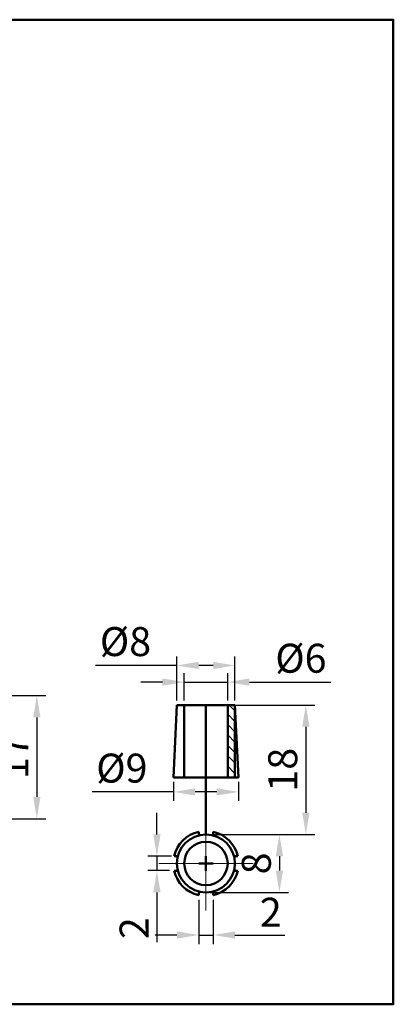
# Model space of a CAD drawing. Units: millimetres. Extents: x 139 to 291, y 28 to 164.
# Tile 5 of 5: x 240 to 291, y 28 to 164. Entities that reach past the tile are written whole.
import ezdxf

# ---------------------------------------------------------------- set-up
doc = ezdxf.new("R2010")
doc.units = ezdxf.units.MM
doc.linetypes.add('CENTER2', pattern=[28.575, 19.05, -3.175, 3.175, -3.175])
for name, color, linetype, lineweight in [('M-CNTR', 1, 'CENTER2', 18), ('M-DIMS', 2, 'Continuous', 25), ('M-HATC', 8, 'Continuous', 18), ('M-OUTL', 7, 'Continuous', 50)]:
    doc.layers.add(name, color=color, linetype=linetype, lineweight=lineweight)
doc.styles.get("Standard").update_dxf_attribs({"font": 'arial.ttf'})
doc.dimstyles.new('ISO-25', dxfattribs={"dimtxt": 4, "dimasz": 3, "dimexe": 1.25, "dimexo": 0.625, "dimtad": 1, "dimdec": 0, "dimtxsty": 'Standard', "dimcen": 2.5, "dimadec": 0, "dimazin": 0, "dimtfac": 1, "dimtdec": 0, "dimtmove": 0, "dimatfit": 3, "dimfxl": 1, "dimarcsym": 0})

# ---------------------------------------------------------------- blocks, each defined once
blk = doc.blocks.new('*D18')
at = {"layer": 'Defpoints', "color": 0, "transparency": 16777216}
for p in [(268.38, 72.71), (262.38, 69.54), (268.38, 69.54)]:
    blk.add_point(p, dxfattribs=at)
at = {"layer": 'M-DIMS', "color": 0, "lineweight": -2, "transparency": 16777216}
for p, q in [((262.38, 70.16), (262.38, 73.96)), ((268.38, 70.16), (268.38, 73.96)), ((259.38, 72.71), (256.38, 72.71)), ((262.38, 72.71), (268.38, 72.71)), ((271.38, 72.71), (282.6, 72.71))]:
    blk.add_line(p, q, dxfattribs=at)
at = {"layer": 'M-DIMS', "color": 0, "transparency": 16777216}
for points in [[(259.38, 73.21), (259.38, 72.21), (262.38, 72.71)], [(271.38, 73.21), (271.38, 72.21), (268.38, 72.71)]]:
    blk.add_solid(points, dxfattribs=at)
at = {"layer": 'M-DIMS', "color": 0, "transparency": 16777216, "insert": (278.49, 75.49), "char_height": 4, "attachment_point": 5}
blk.add_mtext('%%C6', dxfattribs=at)
blk = doc.blocks.new('*D19')
at = {"layer": 'Defpoints', "color": 0, "transparency": 16777216}
for p in [(269.38, 75.01), (261.38, 69.54), (269.38, 69.54)]:
    blk.add_point(p, dxfattribs=at)
at = {"layer": 'M-DIMS', "color": 0, "lineweight": -2, "transparency": 16777216}
for p, q in [((261.38, 70.16), (261.38, 76.26)), ((269.38, 70.16), (269.38, 76.26)), ((261.38, 75.01), (250.15, 75.01)), ((266.38, 75.01), (264.38, 75.01))]:
    blk.add_line(p, q, dxfattribs=at)
at = {"layer": 'M-DIMS', "color": 0, "transparency": 16777216}
for points in [[(264.38, 75.51), (264.38, 74.51), (261.38, 75.01)], [(266.38, 75.51), (266.38, 74.51), (269.38, 75.01)]]:
    blk.add_solid(points, dxfattribs=at)
at = {"layer": 'M-DIMS', "color": 0, "transparency": 16777216, "insert": (254.27, 77.79), "char_height": 4, "attachment_point": 5}
blk.add_mtext('%%C8', dxfattribs=at)
blk = doc.blocks.new('*D20')
at = {"layer": 'Defpoints', "color": 0, "transparency": 16777216}
for p in [(265.38, 69.54), (265.38, 51.66), (279.17, 51.66)]:
    blk.add_point(p, dxfattribs=at)
at = {"layer": 'M-DIMS', "color": 0, "lineweight": -2, "transparency": 16777216}
for p, q in [((266.01, 69.54), (280.42, 69.54)), ((279.17, 66.54), (279.17, 54.66)), ((266.01, 51.66), (280.42, 51.66))]:
    blk.add_line(p, q, dxfattribs=at)
at = {"layer": 'M-DIMS', "color": 0, "transparency": 16777216}
for points in [[(278.67, 66.54), (279.67, 66.54), (279.17, 69.54)], [(278.67, 54.66), (279.67, 54.66), (279.17, 51.66)]]:
    blk.add_solid(points, dxfattribs=at)
at = {"layer": 'M-DIMS', "color": 0, "transparency": 16777216, "insert": (276.5, 60.6), "char_height": 4, "attachment_point": 5, "rotation": 90}
blk.add_mtext('18', dxfattribs=at)
blk = doc.blocks.new('*D21')
at = {"layer": 'Defpoints', "color": 0, "transparency": 16777216}
for p in [(260.88, 59.54), (269.88, 59.54), (269.88, 57.54)]:
    blk.add_point(p, dxfattribs=at)
at = {"layer": 'M-DIMS', "color": 0, "lineweight": -2, "transparency": 16777216}
for p, q in [((260.88, 58.91), (260.88, 56.29)), ((269.88, 58.91), (269.88, 56.29)), ((260.88, 57.54), (249.65, 57.54)), ((266.88, 57.54), (263.88, 57.54))]:
    blk.add_line(p, q, dxfattribs=at)
at = {"layer": 'M-DIMS', "color": 0, "transparency": 16777216}
for points in [[(263.88, 58.04), (263.88, 57.04), (260.88, 57.54)], [(266.88, 58.04), (266.88, 57.04), (269.88, 57.54)]]:
    blk.add_solid(points, dxfattribs=at)
at = {"layer": 'M-DIMS', "color": 0, "transparency": 16777216, "insert": (253.77, 60.31), "char_height": 4, "attachment_point": 5}
blk.add_mtext('%%C9', dxfattribs=at)
blk = doc.blocks.new('*U22')
at = {"layer": 'M-CNTR', "color": 0, "transparency": 16777216}
for p, q in [((0, 0.6), (0, 6.5)), ((-6.5, 0), (-0.6, 0)), ((0.6, 0), (6.5, 0)), ((0, -6.5), (0, -0.6))]:
    blk.add_line(p, q, dxfattribs=at)
at = {"layer": 'M-CNTR', "color": 0, "linetype": 'Continuous', "transparency": 16777216}
for p, q in [((-0.3, 0), (0.3, 0)), ((0, -0.3), (0, 0.3))]:
    blk.add_line(p, q, dxfattribs=at)
blk = doc.blocks.new('*D23')
at = {"layer": 'Defpoints', "color": 0, "transparency": 16777216}
for p in [(265.38, 51.66), (265.38, 43.66), (275.52, 43.66)]:
    blk.add_point(p, dxfattribs=at)
at = {"layer": 'M-DIMS', "color": 0, "lineweight": -2, "transparency": 16777216}
for p, q in [((266.01, 51.66), (276.77, 51.66)), ((275.52, 48.66), (275.52, 46.66)), ((266.01, 43.66), (276.77, 43.66))]:
    blk.add_line(p, q, dxfattribs=at)
at = {"layer": 'M-DIMS', "color": 0, "transparency": 16777216}
for points in [[(275.02, 48.66), (276.02, 48.66), (275.52, 51.66)], [(275.02, 46.66), (276.02, 46.66), (275.52, 43.66)]]:
    blk.add_solid(points, dxfattribs=at)
at = {"layer": 'M-DIMS', "color": 0, "transparency": 16777216, "insert": (272.85, 47.66), "char_height": 4, "attachment_point": 5, "rotation": 90}
blk.add_mtext('8', dxfattribs=at)
blk = doc.blocks.new('*D24')
at = {"layer": 'Defpoints', "color": 0, "transparency": 16777216}
for p in [(264.38, 43.27), (266.38, 43.27), (266.38, 37.77)]:
    blk.add_point(p, dxfattribs=at)
at = {"layer": 'M-DIMS', "color": 0, "lineweight": -2, "transparency": 16777216}
for p, q in [((264.38, 42.64), (264.38, 36.52)), ((266.38, 42.64), (266.38, 36.52)), ((261.38, 37.77), (258.38, 37.77)), ((264.38, 37.77), (266.38, 37.77)), ((269.38, 37.77), (276.28, 37.77))]:
    blk.add_line(p, q, dxfattribs=at)
at = {"layer": 'M-DIMS', "color": 0, "transparency": 16777216}
for points in [[(261.38, 38.27), (261.38, 37.27), (264.38, 37.77)], [(269.38, 38.27), (269.38, 37.27), (266.38, 37.77)]]:
    blk.add_solid(points, dxfattribs=at)
at = {"layer": 'M-DIMS', "color": 0, "transparency": 16777216, "insert": (274.33, 40.4), "char_height": 4, "attachment_point": 5}
blk.add_mtext('2', dxfattribs=at)
blk = doc.blocks.new('*D25')
at = {"layer": 'Defpoints', "color": 0, "transparency": 16777216}
for p in [(261.25, 48.66), (258.61, 46.66), (261, 46.66)]:
    blk.add_point(p, dxfattribs=at)
at = {"layer": 'M-DIMS', "color": 0, "lineweight": -2, "transparency": 16777216}
for p, q in [((258.61, 51.66), (258.61, 54.66)), ((260.63, 48.66), (257.36, 48.66)), ((258.61, 48.66), (258.61, 46.66)), ((260.37, 46.66), (257.36, 46.66)), ((258.61, 43.66), (258.61, 36.76))]:
    blk.add_line(p, q, dxfattribs=at)
at = {"layer": 'M-DIMS', "color": 0, "transparency": 16777216}
for points in [[(258.11, 51.66), (259.11, 51.66), (258.61, 48.66)], [(258.11, 43.66), (259.11, 43.66), (258.61, 46.66)]]:
    blk.add_solid(points, dxfattribs=at)
at = {"layer": 'M-DIMS', "color": 0, "transparency": 16777216, "insert": (255.98, 38.71), "char_height": 4, "attachment_point": 5, "rotation": 90}
blk.add_mtext('2', dxfattribs=at)
blk = doc.blocks.new('*D31')
at = {"layer": 'Defpoints', "color": 0, "transparency": 16777216}
for p in [(229.29, 70.84), (229.29, 53.84), (242.03, 53.84)]:
    blk.add_point(p, dxfattribs=at)
at = {"layer": 'M-DIMS', "color": 0, "lineweight": -2, "transparency": 16777216}
for p, q in [((229.91, 70.84), (243.28, 70.84)), ((242.03, 67.84), (242.03, 56.84)), ((229.91, 53.84), (243.28, 53.84))]:
    blk.add_line(p, q, dxfattribs=at)
at = {"layer": 'M-DIMS', "color": 0, "transparency": 16777216}
for points in [[(241.53, 67.84), (242.53, 67.84), (242.03, 70.84)], [(241.53, 56.84), (242.53, 56.84), (242.03, 53.84)]]:
    blk.add_solid(points, dxfattribs=at)
at = {"layer": 'M-DIMS', "color": 0, "transparency": 16777216, "insert": (239.4, 62.34), "char_height": 4, "attachment_point": 5, "rotation": 90}
blk.add_mtext('17', dxfattribs=at)

msp = doc.modelspace()

# ---------------------------------------------------------------- hatches: boundary and pattern name
at = {"layer": 'M-HATC'}
h = msp.add_hatch(dxfattribs=at)
h.set_pattern_fill('ANSI31', color=256, scale=0.32, angle=90)
h.set_pattern_definition([(135, (8.7224, -45.6361), (-0.7184205, -0.7184205), [])])
h.paths.add_polyline_path([(269.3825, 69.5382), (268.3825, 69.5382), (268.3825, 59.5382), (269.3825, 59.5382)])

# ---------------------------------------------------------------- linework, layer by layer
at = {"layer": 'M-OUTL'}
for p, q in [((261.3825, 69.5382), (260.8825, 59.5382)), ((261.3825, 69.5382), (269.3825, 69.5382)), ((262.3825, 59.5382), (262.3825, 69.5382)), ((265.3825, 51.6573), (265.3825, 69.5382)), ((268.3825, 59.5382), (268.3825, 69.5382)), ((269.3825, 69.5382), (269.8825, 59.5382)), ((269.3825, 69.5382), (269.3825, 59.5382)), ((260.8825, 59.5382), (269.8825, 59.5382)), ((264.3825, 51.5303), (264.3825, 52.0448)), ((266.3825, 52.0448), (266.3825, 51.5303)), ((260.995, 48.6573), (261.5095, 48.6573)), ((264.3825, 47.6573), (266.3825, 47.6573)), ((265.3825, 48.6573), (265.3825, 46.6573)), ((269.2555, 48.6573), (269.77, 48.6573)), ((261.5095, 46.6573), (260.995, 46.6573)), ((269.77, 46.6573), (269.2555, 46.6573)), ((264.3825, 43.2698), (264.3825, 43.7843)), ((266.3825, 43.7843), (266.3825, 43.2698))]:
    msp.add_line(p, q, dxfattribs=at)
msp.add_lwpolyline([(139.74, 164.2339), (291.244, 164.2339), (291.244, 28.1944), (139.74, 28.1944)], close=True, dxfattribs=at)
for radius in [4, 3]:
    msp.add_circle((265.3825, 47.6573), radius, dxfattribs=at)
for start, end in [(102.839588, 167.160412), (12.839588, 77.160412), (192.839588, 257.160412), (282.839588, 347.160412)]:
    msp.add_arc((265.3825, 47.6573), 4.5, start, end, dxfattribs=at)

# ---------------------------------------------------------------- block references
at = {"layer": 'M-CNTR'}
msp.add_blockref('*U22', (265.3825, 47.6573), dxfattribs=at)

# ---------------------------------------------------------------- dimensions: what is measured, and where the dimension line sits
at = {"layer": 'M-DIMS'}
for base, p1, p2, picture, middle in [((269.3825, 75.006), (261.3825, 69.5382), (269.3825, 69.5382), '*D19', (254.2664, 75.006)), ((269.8825, 57.5353), (260.8825, 59.5382), (269.8825, 59.5382), '*D21', (253.7664, 57.5353))]:
    dim = msp.add_linear_dim(base=base, p1=p1, p2=p2, text='%%C<>', dimstyle='ISO-25', override={"dimclrd": 0, "dimclre": 0, "dimclrt": 0}, dxfattribs=at)
    dim.commit()
    dim.dimension.update_dxf_attribs({"geometry": picture, "text_midpoint": middle, "dimtype": 160})
dim = msp.add_linear_dim(base=(268.3825, 72.7059), p1=(262.3825, 69.5382), p2=(268.3825, 69.5382), text='%%C<>', dimstyle='ISO-25', override={"dimclrd": 0, "dimclre": 0, "dimclrt": 0}, dxfattribs=at)
dim.commit()
dim.dimension.update_dxf_attribs({"geometry": '*D18', "text_midpoint": (278.4932, 75.4851)})
for base, p1, p2, picture, middle in [((242.0317, 53.8364), (229.2871, 70.8364), (229.2871, 53.8364), '*D31', (239.3985, 62.3364)), ((279.1664, 51.6573), (265.3825, 69.5382), (265.3825, 51.6573), '*D20', (276.4991, 60.5977)), ((258.6096, 46.6573), (261.2523, 48.6573), (260.995, 46.6573), '*D25', (255.9764, 38.7076)), ((275.521, 43.6573), (265.3825, 51.6573), (265.3825, 43.6573), '*D23', (272.8537, 47.6573))]:
    dim = msp.add_linear_dim(base=base, p1=p1, p2=p2, angle=90, dimstyle='ISO-25', override={"dimclrd": 0, "dimclre": 0, "dimclrt": 0}, dxfattribs=at)
    dim.commit()
    dim.dimension.update_dxf_attribs({"geometry": picture, "text_midpoint": middle})
dim = msp.add_linear_dim(base=(266.3825, 37.7711), p1=(264.3825, 43.2698), p2=(266.3825, 43.2698), dimstyle='ISO-25', override={"dimclrd": 0, "dimclre": 0, "dimclrt": 0}, dxfattribs=at)
dim.commit()
dim.dimension.update_dxf_attribs({"geometry": '*D24', "text_midpoint": (274.3322, 40.4043)})

doc.saveas('drawing.dxf')
